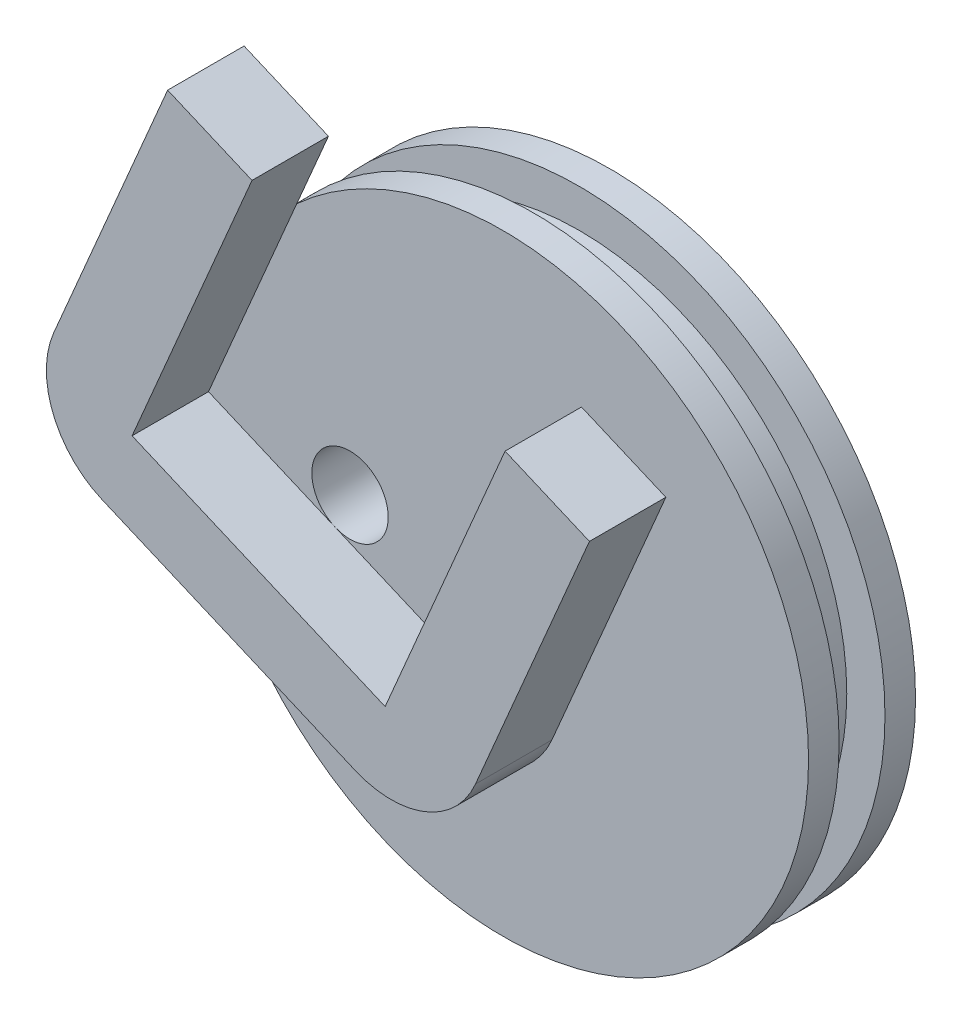
ISO-10303-21;
HEADER;
FILE_DESCRIPTION(('STEP AP214'),'2;1');
FILE_NAME('part.step','',(''),(''),'','','');
FILE_SCHEMA(('AUTOMOTIVE_DESIGN { 1 0 10303 214 1 1 1 1 }'));
ENDSEC;
DATA;
#1=APPLICATION_CONTEXT('core data for automotive mechanical design processes');
#2=APPLICATION_PROTOCOL_DEFINITION('international standard','automotive_design',2000,#1);
#3=PRODUCT_CONTEXT('',#1,'mechanical');
#4=PRODUCT('Part','Part','',(#3));
#5=PRODUCT_RELATED_PRODUCT_CATEGORY('part','',(#4));
#6=PRODUCT_DEFINITION_FORMATION('','',#4);
#7=PRODUCT_DEFINITION_CONTEXT('part definition',#1,'design');
#8=PRODUCT_DEFINITION('design','',#6,#7);
#9=PRODUCT_DEFINITION_SHAPE('','',#8);
#10=(LENGTH_UNIT() NAMED_UNIT(*) SI_UNIT(.MILLI.,.METRE.));
#11=(NAMED_UNIT(*) PLANE_ANGLE_UNIT() SI_UNIT($,.RADIAN.));
#12=(NAMED_UNIT(*) SI_UNIT($,.STERADIAN.) SOLID_ANGLE_UNIT());
#13=UNCERTAINTY_MEASURE_WITH_UNIT(LENGTH_MEASURE(1.E-05),#10,'distance_accuracy_value','');
#14=(GEOMETRIC_REPRESENTATION_CONTEXT(3) GLOBAL_UNCERTAINTY_ASSIGNED_CONTEXT((#13)) GLOBAL_UNIT_ASSIGNED_CONTEXT((#10,
#11,#12)) REPRESENTATION_CONTEXT('',''));
#15=CARTESIAN_POINT('',(0.,0.,0.));
#16=DIRECTION('',(0.,0.,1.));
#17=DIRECTION('',(1.,0.,0.));
#18=AXIS2_PLACEMENT_3D('',#15,#16,#17);
#19=CARTESIAN_POINT('',(0.,0.,3.5));
#20=DIRECTION('',(0.,0.,-1.));
#21=DIRECTION('',(-1.,0.,0.));
#22=AXIS2_PLACEMENT_3D('',#19,#20,#21);
#23=CYLINDRICAL_SURFACE('',#22,20.);
#24=CARTESIAN_POINT('',(0.,0.,3.5));
#25=DIRECTION('',(0.,0.,1.));
#26=DIRECTION('',(1.,0.,0.));
#27=AXIS2_PLACEMENT_3D('',#24,#25,#26);
#28=CIRCLE('',#27,20.);
#29=CARTESIAN_POINT('',(-13.4841723935684,14.7708190314731,3.5));
#30=VERTEX_POINT('',#29);
#31=CARTESIAN_POINT('',(-19.5822117840181,-4.06656878041691,3.5));
#32=VERTEX_POINT('',#31);
#33=EDGE_CURVE('E229',#30,#32,#28,.T.);
#34=ORIENTED_EDGE('',*,*,#33,.F.);
#35=EDGE_CURVE('E226',#32,#30,#28,.T.);
#36=ORIENTED_EDGE('',*,*,#35,.F.);
#37=EDGE_LOOP('',(#34,#36));
#38=FACE_BOUND('',#37,.T.);
#39=CARTESIAN_POINT('',(0.,0.,1.5));
#40=DIRECTION('',(0.,0.,1.));
#41=DIRECTION('',(1.,0.,0.));
#42=AXIS2_PLACEMENT_3D('',#39,#40,#41);
#43=CIRCLE('',#42,20.);
#44=CARTESIAN_POINT('',(20.,0.,1.5));
#45=VERTEX_POINT('',#44);
#46=EDGE_CURVE('E212',#45,#45,#43,.T.);
#47=ORIENTED_EDGE('',*,*,#46,.T.);
#48=EDGE_LOOP('',(#47));
#49=FACE_BOUND('',#48,.T.);
#50=ADVANCED_FACE('F39',(#38,#49),#23,.T.);
#51=CARTESIAN_POINT('',(0.,0.,3.5));
#52=DIRECTION('',(0.,0.,1.));
#53=DIRECTION('',(1.,0.,0.));
#54=AXIS2_PLACEMENT_3D('',#51,#52,#53);
#55=PLANE('',#54);
#56=DIRECTION('',(0.39234033710411,0.919820123655181,0.));
#57=VECTOR('',#56,1.);
#58=CARTESIAN_POINT('',(-19.2592319556569,1.231512724799,3.5));
#59=LINE('',#58,#57);
#60=CARTESIAN_POINT('',(-19.2592319556569,1.231512724799,3.5));
#61=VERTEX_POINT('',#60);
#62=EDGE_CURVE('E60',#61,#30,#59,.T.);
#63=ORIENTED_EDGE('',*,*,#62,.F.);
#64=DIRECTION('',(0.919820123655183,-0.392340337104106,0.));
#65=VECTOR('',#64,1.);
#66=CARTESIAN_POINT('',(-19.2592319556569,1.231512724799,3.5));
#67=LINE('',#66,#65);
#68=CARTESIAN_POINT('',(-10.9808508427603,-2.29955030913796,3.5));
#69=VERTEX_POINT('',#68);
#70=EDGE_CURVE('E49',#61,#69,#67,.T.);
#71=ORIENTED_EDGE('',*,*,#70,.T.);
#72=CARTESIAN_POINT('',(-10.,0.,3.5));
#73=DIRECTION('',(0.,0.,1.));
#74=DIRECTION('',(1.,0.,0.));
#75=AXIS2_PLACEMENT_3D('',#72,#73,#74);
#76=CIRCLE('',#75,2.5);
#77=EDGE_CURVE('E192',#69,#69,#76,.T.);
#78=ORIENTED_EDGE('',*,*,#77,.F.);
#79=CARTESIAN_POINT('',(-2.70246972986364,-5.8306133430749,3.5));
#80=VERTEX_POINT('',#79);
#81=EDGE_CURVE('E11',#69,#80,#67,.T.);
#82=ORIENTED_EDGE('',*,*,#81,.T.);
#83=DIRECTION('',(0.392340337104111,0.919820123655181,0.));
#84=VECTOR('',#83,1.);
#85=CARTESIAN_POINT('',(-2.70246972986364,-5.8306133430749,3.5));
#86=LINE('',#85,#84);
#87=CARTESIAN_POINT('',(5.14433701221858,12.5657891300287,3.5));
#88=VERTEX_POINT('',#87);
#89=EDGE_CURVE('E182',#80,#88,#86,.T.);
#90=ORIENTED_EDGE('',*,*,#89,.T.);
#91=DIRECTION('',(0.919820123655182,-0.392340337104108,0.));
#92=VECTOR('',#91,1.);
#93=CARTESIAN_POINT('',(5.14433701221858,12.5657891300287,3.5));
#94=LINE('',#93,#92);
#95=CARTESIAN_POINT('',(10.6632577541501,10.2117471074039,3.5));
#96=VERTEX_POINT('',#95);
#97=EDGE_CURVE('E181',#88,#96,#94,.T.);
#98=ORIENTED_EDGE('',*,*,#97,.T.);
#99=DIRECTION('',(0.392340337104132,0.919820123655172,0.));
#100=VECTOR('',#99,1.);
#101=CARTESIAN_POINT('',(3.20879134917148,-7.2648352420445,3.5));
#102=LINE('',#101,#100);
#103=CARTESIAN_POINT('',(3.2087913491715,-7.26483524204451,3.5));
#104=VERTEX_POINT('',#103);
#105=EDGE_CURVE('E183',#104,#96,#102,.T.);
#106=ORIENTED_EDGE('',*,*,#105,.F.);
#107=CARTESIAN_POINT('',(-2.31012939275951,-4.91079321941972,3.5));
#108=DIRECTION('',(0.,0.,1.));
#109=DIRECTION('',(1.,0.,0.));
#110=AXIS2_PLACEMENT_3D('',#107,#108,#109);
#111=CIRCLE('',#110,5.99999999999998);
#112=CARTESIAN_POINT('',(-4.66417141538418,-10.4297139613508,3.5));
#113=VERTEX_POINT('',#112);
#114=EDGE_CURVE('E153',#113,#104,#111,.T.);
#115=ORIENTED_EDGE('',*,*,#114,.F.);
#116=DIRECTION('',(0.919820123655183,-0.392340337104106,0.));
#117=VECTOR('',#116,1.);
#118=CARTESIAN_POINT('',(-21.2209336411774,-3.36758789347694,3.5));
#119=LINE('',#118,#117);
#120=EDGE_CURVE('E48',#32,#113,#119,.T.);
#121=ORIENTED_EDGE('',*,*,#120,.F.);
#122=ORIENTED_EDGE('',*,*,#35,.T.);
#123=EDGE_LOOP('',(#63,#71,#78,#82,#90,#98,#106,#115,#121,#122));
#124=FACE_BOUND('',#123,.T.);
#125=ADVANCED_FACE('F233',(#124),#55,.T.);
#126=CARTESIAN_POINT('',(0.,20.,1.5));
#127=DIRECTION('',(0.,0.,-1.));
#128=DIRECTION('',(-1.,0.,0.));
#129=AXIS2_PLACEMENT_3D('',#126,#127,#128);
#130=PLANE('',#129);
#131=CARTESIAN_POINT('',(0.,0.,1.5));
#132=DIRECTION('',(0.,0.,1.));
#133=DIRECTION('',(1.,0.,0.));
#134=AXIS2_PLACEMENT_3D('',#131,#132,#133);
#135=CIRCLE('',#134,17.5);
#136=CARTESIAN_POINT('',(17.5,0.,1.5));
#137=VERTEX_POINT('',#136);
#138=EDGE_CURVE('E224',#137,#137,#135,.T.);
#139=ORIENTED_EDGE('',*,*,#138,.T.);
#140=EDGE_LOOP('',(#139));
#141=FACE_BOUND('',#140,.T.);
#142=ORIENTED_EDGE('',*,*,#46,.F.);
#143=EDGE_LOOP('',(#142));
#144=FACE_BOUND('',#143,.T.);
#145=ADVANCED_FACE('F280',(#141,#144),#130,.T.);
#146=CARTESIAN_POINT('',(0.,0.,14.756637322569));
#147=DIRECTION('',(0.,0.,1.));
#148=DIRECTION('',(1.,0.,0.));
#149=AXIS2_PLACEMENT_3D('',#146,#147,#148);
#150=CYLINDRICAL_SURFACE('',#149,17.5);
#151=CARTESIAN_POINT('',(0.,0.,-1.5));
#152=DIRECTION('',(0.,0.,1.));
#153=DIRECTION('',(1.,0.,0.));
#154=AXIS2_PLACEMENT_3D('',#151,#152,#153);
#155=CIRCLE('',#154,17.5);
#156=CARTESIAN_POINT('',(17.5,0.,-1.5));
#157=VERTEX_POINT('',#156);
#158=EDGE_CURVE('E219',#157,#157,#155,.T.);
#159=ORIENTED_EDGE('',*,*,#158,.T.);
#160=EDGE_LOOP('',(#159));
#161=FACE_BOUND('',#160,.T.);
#162=ORIENTED_EDGE('',*,*,#138,.F.);
#163=EDGE_LOOP('',(#162));
#164=FACE_BOUND('',#163,.T.);
#165=ADVANCED_FACE('F269',(#161,#164),#150,.T.);
#166=CARTESIAN_POINT('',(0.,20.,-1.5));
#167=DIRECTION('',(0.,0.,-1.));
#168=DIRECTION('',(-1.,0.,0.));
#169=AXIS2_PLACEMENT_3D('',#166,#167,#168);
#170=PLANE('',#169);
#171=ORIENTED_EDGE('',*,*,#158,.F.);
#172=EDGE_LOOP('',(#171));
#173=FACE_BOUND('',#172,.T.);
#174=CARTESIAN_POINT('',(0.,0.,-1.5));
#175=DIRECTION('',(0.,0.,1.));
#176=DIRECTION('',(1.,0.,0.));
#177=AXIS2_PLACEMENT_3D('',#174,#175,#176);
#178=CIRCLE('',#177,20.);
#179=CARTESIAN_POINT('',(20.,0.,-1.5));
#180=VERTEX_POINT('',#179);
#181=EDGE_CURVE('E220',#180,#180,#178,.T.);
#182=ORIENTED_EDGE('',*,*,#181,.T.);
#183=EDGE_LOOP('',(#182));
#184=FACE_BOUND('',#183,.T.);
#185=ADVANCED_FACE('F263',(#173,#184),#170,.F.);
#186=CARTESIAN_POINT('',(0.,0.,-3.5));
#187=DIRECTION('',(0.,0.,1.));
#188=DIRECTION('',(1.,0.,0.));
#189=AXIS2_PLACEMENT_3D('',#186,#187,#188);
#190=PLANE('',#189);
#191=CARTESIAN_POINT('',(-10.,0.,-3.5));
#192=DIRECTION('',(0.,0.,1.));
#193=DIRECTION('',(1.,0.,0.));
#194=AXIS2_PLACEMENT_3D('',#191,#192,#193);
#195=CIRCLE('',#194,2.5);
#196=CARTESIAN_POINT('',(-7.5,0.,-3.5));
#197=VERTEX_POINT('',#196);
#198=EDGE_CURVE('E43',#197,#197,#195,.T.);
#199=ORIENTED_EDGE('',*,*,#198,.T.);
#200=EDGE_LOOP('',(#199));
#201=FACE_BOUND('',#200,.T.);
#202=CARTESIAN_POINT('',(0.,0.,-3.5));
#203=DIRECTION('',(0.,0.,1.));
#204=DIRECTION('',(1.,0.,0.));
#205=AXIS2_PLACEMENT_3D('',#202,#203,#204);
#206=CIRCLE('',#205,20.);
#207=CARTESIAN_POINT('',(20.,0.,-3.5));
#208=VERTEX_POINT('',#207);
#209=EDGE_CURVE('E227',#208,#208,#206,.T.);
#210=ORIENTED_EDGE('',*,*,#209,.F.);
#211=EDGE_LOOP('',(#210));
#212=FACE_BOUND('',#211,.T.);
#213=ADVANCED_FACE('F257',(#201,#212),#190,.F.);
#214=ORIENTED_EDGE('',*,*,#181,.F.);
#215=EDGE_LOOP('',(#214));
#216=FACE_BOUND('',#215,.T.);
#217=ORIENTED_EDGE('',*,*,#209,.T.);
#218=EDGE_LOOP('',(#217));
#219=FACE_BOUND('',#218,.T.);
#220=ADVANCED_FACE('F41',(#216,#219),#23,.T.);
#221=CARTESIAN_POINT('',(-10.,0.,-43.5));
#222=DIRECTION('',(0.,0.,1.));
#223=DIRECTION('',(1.,0.,0.));
#224=AXIS2_PLACEMENT_3D('',#221,#222,#223);
#225=CYLINDRICAL_SURFACE('',#224,2.5);
#226=ORIENTED_EDGE('',*,*,#77,.T.);
#227=EDGE_LOOP('',(#226));
#228=FACE_BOUND('',#227,.T.);
#229=ORIENTED_EDGE('',*,*,#198,.F.);
#230=EDGE_LOOP('',(#229));
#231=FACE_BOUND('',#230,.T.);
#232=ADVANCED_FACE('F251',(#228,#231),#225,.F.);
#233=CARTESIAN_POINT('',(-18.8668916185528,2.15133284845418,8.5));
#234=DIRECTION('',(0.,0.,-1.));
#235=DIRECTION('',(-1.,0.,0.));
#236=AXIS2_PLACEMENT_3D('',#233,#234,#235);
#237=CYLINDRICAL_SURFACE('',#236,6.00000000000002);
#238=CARTESIAN_POINT('',(-18.8668916185528,2.15133284845418,3.5));
#239=DIRECTION('',(0.,0.,-1.));
#240=DIRECTION('',(-1.,0.,0.));
#241=AXIS2_PLACEMENT_3D('',#238,#239,#240);
#242=CIRCLE('',#241,6.00000000000002);
#243=CARTESIAN_POINT('',(-21.2209336411774,-3.36758789347694,3.5));
#244=VERTEX_POINT('',#243);
#245=CARTESIAN_POINT('',(-24.3858123604839,4.505374871079,3.5));
#246=VERTEX_POINT('',#245);
#247=EDGE_CURVE('E175',#244,#246,#242,.T.);
#248=ORIENTED_EDGE('',*,*,#247,.F.);
#249=DIRECTION('',(0.,0.,-1.));
#250=VECTOR('',#249,1.);
#251=CARTESIAN_POINT('',(-21.2209336411774,-3.36758789347694,8.5));
#252=LINE('',#251,#250);
#253=CARTESIAN_POINT('',(-21.2209336411774,-3.36758789347694,8.5));
#254=VERTEX_POINT('',#253);
#255=EDGE_CURVE('E146',#254,#244,#252,.T.);
#256=ORIENTED_EDGE('',*,*,#255,.F.);
#257=CARTESIAN_POINT('',(-18.8668916185528,2.15133284845418,8.5));
#258=DIRECTION('',(0.,0.,-1.));
#259=DIRECTION('',(-1.,0.,0.));
#260=AXIS2_PLACEMENT_3D('',#257,#258,#259);
#261=CIRCLE('',#260,6.00000000000002);
#262=CARTESIAN_POINT('',(-24.3858123604839,4.505374871079,8.5));
#263=VERTEX_POINT('',#262);
#264=EDGE_CURVE('E141',#254,#263,#261,.T.);
#265=ORIENTED_EDGE('',*,*,#264,.T.);
#266=DIRECTION('',(0.,0.,-1.));
#267=VECTOR('',#266,1.);
#268=CARTESIAN_POINT('',(-24.3858123604839,4.505374871079,8.5));
#269=LINE('',#268,#267);
#270=EDGE_CURVE('E127',#263,#246,#269,.T.);
#271=ORIENTED_EDGE('',*,*,#270,.T.);
#272=EDGE_LOOP('',(#248,#256,#265,#271));
#273=FACE_BOUND('',#272,.T.);
#274=ADVANCED_FACE('F150',(#273),#237,.T.);
#275=CARTESIAN_POINT('',(-21.2209336411774,-3.36758789347694,8.5));
#276=DIRECTION('',(0.392340337104106,0.919820123655183,0.));
#277=DIRECTION('',(-0.919820123655183,0.392340337104106,0.));
#278=AXIS2_PLACEMENT_3D('',#275,#276,#277);
#279=PLANE('',#278);
#280=EDGE_CURVE('E147',#244,#32,#119,.T.);
#281=ORIENTED_EDGE('',*,*,#280,.T.);
#282=ORIENTED_EDGE('',*,*,#120,.T.);
#283=DIRECTION('',(0.,0.,-1.));
#284=VECTOR('',#283,1.);
#285=CARTESIAN_POINT('',(-4.66417141538418,-10.4297139613508,8.5));
#286=LINE('',#285,#284);
#287=CARTESIAN_POINT('',(-4.66417141538418,-10.4297139613508,8.5));
#288=VERTEX_POINT('',#287);
#289=EDGE_CURVE('E194',#288,#113,#286,.T.);
#290=ORIENTED_EDGE('',*,*,#289,.F.);
#291=DIRECTION('',(0.919820123655183,-0.392340337104106,0.));
#292=VECTOR('',#291,1.);
#293=CARTESIAN_POINT('',(-21.2209336411774,-3.36758789347694,8.5));
#294=LINE('',#293,#292);
#295=EDGE_CURVE('E139',#254,#288,#294,.T.);
#296=ORIENTED_EDGE('',*,*,#295,.F.);
#297=ORIENTED_EDGE('',*,*,#255,.T.);
#298=EDGE_LOOP('',(#281,#282,#290,#296,#297));
#299=FACE_BOUND('',#298,.T.);
#300=ADVANCED_FACE('F286',(#299),#279,.F.);
#301=CARTESIAN_POINT('',(-2.31012939275951,-4.91079321941972,8.5));
#302=DIRECTION('',(0.,0.,-1.));
#303=DIRECTION('',(-1.,0.,0.));
#304=AXIS2_PLACEMENT_3D('',#301,#302,#303);
#305=CYLINDRICAL_SURFACE('',#304,5.99999999999998);
#306=ORIENTED_EDGE('',*,*,#114,.T.);
#307=DIRECTION('',(0.,0.,-1.));
#308=VECTOR('',#307,1.);
#309=CARTESIAN_POINT('',(3.2087913491715,-7.26483524204451,8.5));
#310=LINE('',#309,#308);
#311=CARTESIAN_POINT('',(3.2087913491715,-7.26483524204451,8.5));
#312=VERTEX_POINT('',#311);
#313=EDGE_CURVE('E193',#312,#104,#310,.T.);
#314=ORIENTED_EDGE('',*,*,#313,.F.);
#315=CARTESIAN_POINT('',(-2.31012939275951,-4.91079321941972,8.5));
#316=DIRECTION('',(0.,0.,1.));
#317=DIRECTION('',(1.,0.,0.));
#318=AXIS2_PLACEMENT_3D('',#315,#316,#317);
#319=CIRCLE('',#318,5.99999999999998);
#320=EDGE_CURVE('E168',#288,#312,#319,.T.);
#321=ORIENTED_EDGE('',*,*,#320,.F.);
#322=ORIENTED_EDGE('',*,*,#289,.T.);
#323=EDGE_LOOP('',(#306,#314,#321,#322));
#324=FACE_BOUND('',#323,.T.);
#325=ADVANCED_FACE('F313',(#324),#305,.T.);
#326=CARTESIAN_POINT('',(3.20879134917148,-7.2648352420445,8.5));
#327=DIRECTION('',(-0.919820123655172,0.392340337104132,0.));
#328=DIRECTION('',(-0.392340337104132,-0.919820123655172,0.));
#329=AXIS2_PLACEMENT_3D('',#326,#327,#328);
#330=PLANE('',#329);
#331=ORIENTED_EDGE('',*,*,#105,.T.);
#332=DIRECTION('',(0.,0.,-1.));
#333=VECTOR('',#332,1.);
#334=CARTESIAN_POINT('',(10.6632577541501,10.2117471074039,8.5));
#335=LINE('',#334,#333);
#336=CARTESIAN_POINT('',(10.6632577541501,10.2117471074039,8.5));
#337=VERTEX_POINT('',#336);
#338=EDGE_CURVE('E196',#337,#96,#335,.T.);
#339=ORIENTED_EDGE('',*,*,#338,.F.);
#340=DIRECTION('',(0.392340337104132,0.919820123655172,0.));
#341=VECTOR('',#340,1.);
#342=CARTESIAN_POINT('',(3.20879134917148,-7.2648352420445,8.5));
#343=LINE('',#342,#341);
#344=EDGE_CURVE('E169',#312,#337,#343,.T.);
#345=ORIENTED_EDGE('',*,*,#344,.F.);
#346=ORIENTED_EDGE('',*,*,#313,.T.);
#347=EDGE_LOOP('',(#331,#339,#345,#346));
#348=FACE_BOUND('',#347,.T.);
#349=ADVANCED_FACE('F307',(#348),#330,.F.);
#350=CARTESIAN_POINT('',(5.14433701221858,12.5657891300287,8.5));
#351=DIRECTION('',(0.392340337104108,0.919820123655182,0.));
#352=DIRECTION('',(-0.919820123655182,0.392340337104108,0.));
#353=AXIS2_PLACEMENT_3D('',#350,#351,#352);
#354=PLANE('',#353);
#355=ORIENTED_EDGE('',*,*,#97,.F.);
#356=DIRECTION('',(0.,0.,-1.));
#357=VECTOR('',#356,1.);
#358=CARTESIAN_POINT('',(5.14433701221858,12.5657891300287,8.5));
#359=LINE('',#358,#357);
#360=CARTESIAN_POINT('',(5.14433701221858,12.5657891300287,8.5));
#361=VERTEX_POINT('',#360);
#362=EDGE_CURVE('E203',#361,#88,#359,.T.);
#363=ORIENTED_EDGE('',*,*,#362,.F.);
#364=DIRECTION('',(0.919820123655182,-0.392340337104108,0.));
#365=VECTOR('',#364,1.);
#366=CARTESIAN_POINT('',(5.14433701221858,12.5657891300287,8.5));
#367=LINE('',#366,#365);
#368=EDGE_CURVE('E164',#361,#337,#367,.T.);
#369=ORIENTED_EDGE('',*,*,#368,.T.);
#370=ORIENTED_EDGE('',*,*,#338,.T.);
#371=EDGE_LOOP('',(#355,#363,#369,#370));
#372=FACE_BOUND('',#371,.T.);
#373=ADVANCED_FACE('F305',(#372),#354,.T.);
#374=CARTESIAN_POINT('',(-2.70246972986364,-5.8306133430749,8.5));
#375=DIRECTION('',(-0.919820123655181,0.392340337104111,0.));
#376=DIRECTION('',(-0.392340337104111,-0.919820123655181,0.));
#377=AXIS2_PLACEMENT_3D('',#374,#375,#376);
#378=PLANE('',#377);
#379=ORIENTED_EDGE('',*,*,#89,.F.);
#380=DIRECTION('',(0.,0.,-1.));
#381=VECTOR('',#380,1.);
#382=CARTESIAN_POINT('',(-2.70246972986364,-5.8306133430749,8.5));
#383=LINE('',#382,#381);
#384=CARTESIAN_POINT('',(-2.70246972986364,-5.8306133430749,8.5));
#385=VERTEX_POINT('',#384);
#386=EDGE_CURVE('E204',#385,#80,#383,.T.);
#387=ORIENTED_EDGE('',*,*,#386,.F.);
#388=DIRECTION('',(0.392340337104111,0.919820123655181,0.));
#389=VECTOR('',#388,1.);
#390=CARTESIAN_POINT('',(-2.70246972986364,-5.8306133430749,8.5));
#391=LINE('',#390,#389);
#392=EDGE_CURVE('E165',#385,#361,#391,.T.);
#393=ORIENTED_EDGE('',*,*,#392,.T.);
#394=ORIENTED_EDGE('',*,*,#362,.T.);
#395=EDGE_LOOP('',(#379,#387,#393,#394));
#396=FACE_BOUND('',#395,.T.);
#397=ADVANCED_FACE('F298',(#396),#378,.T.);
#398=CARTESIAN_POINT('',(-19.2592319556569,1.231512724799,8.5));
#399=DIRECTION('',(0.392340337104106,0.919820123655183,0.));
#400=DIRECTION('',(-0.919820123655183,0.392340337104106,0.));
#401=AXIS2_PLACEMENT_3D('',#398,#399,#400);
#402=PLANE('',#401);
#403=ORIENTED_EDGE('',*,*,#70,.F.);
#404=DIRECTION('',(0.,0.,-1.));
#405=VECTOR('',#404,1.);
#406=CARTESIAN_POINT('',(-19.2592319556569,1.231512724799,8.5));
#407=LINE('',#406,#405);
#408=CARTESIAN_POINT('',(-19.2592319556569,1.231512724799,8.5));
#409=VERTEX_POINT('',#408);
#410=EDGE_CURVE('E206',#409,#61,#407,.T.);
#411=ORIENTED_EDGE('',*,*,#410,.F.);
#412=DIRECTION('',(0.919820123655183,-0.392340337104106,0.));
#413=VECTOR('',#412,1.);
#414=CARTESIAN_POINT('',(-19.2592319556569,1.231512724799,8.5));
#415=LINE('',#414,#413);
#416=EDGE_CURVE('E157',#409,#385,#415,.T.);
#417=ORIENTED_EDGE('',*,*,#416,.T.);
#418=ORIENTED_EDGE('',*,*,#386,.T.);
#419=ORIENTED_EDGE('',*,*,#81,.F.);
#420=EDGE_LOOP('',(#403,#411,#417,#418,#419));
#421=FACE_BOUND('',#420,.T.);
#422=ADVANCED_FACE('F253',(#421),#402,.T.);
#423=CARTESIAN_POINT('',(-19.2592319556569,1.231512724799,8.5));
#424=DIRECTION('',(-0.919820123655181,0.39234033710411,0.));
#425=DIRECTION('',(-0.39234033710411,-0.919820123655181,0.));
#426=AXIS2_PLACEMENT_3D('',#423,#424,#425);
#427=PLANE('',#426);
#428=ORIENTED_EDGE('',*,*,#62,.T.);
#429=CARTESIAN_POINT('',(-11.4124252135747,19.6279151979026,3.5));
#430=VERTEX_POINT('',#429);
#431=EDGE_CURVE('E176',#30,#430,#59,.T.);
#432=ORIENTED_EDGE('',*,*,#431,.T.);
#433=DIRECTION('',(0.,0.,-1.));
#434=VECTOR('',#433,1.);
#435=CARTESIAN_POINT('',(-11.4124252135747,19.6279151979026,8.5));
#436=LINE('',#435,#434);
#437=CARTESIAN_POINT('',(-11.4124252135747,19.6279151979026,8.5));
#438=VERTEX_POINT('',#437);
#439=EDGE_CURVE('E208',#438,#430,#436,.T.);
#440=ORIENTED_EDGE('',*,*,#439,.F.);
#441=DIRECTION('',(0.39234033710411,0.919820123655181,0.));
#442=VECTOR('',#441,1.);
#443=CARTESIAN_POINT('',(-19.2592319556569,1.231512724799,8.5));
#444=LINE('',#443,#442);
#445=EDGE_CURVE('E160',#409,#438,#444,.T.);
#446=ORIENTED_EDGE('',*,*,#445,.F.);
#447=ORIENTED_EDGE('',*,*,#410,.T.);
#448=EDGE_LOOP('',(#428,#432,#440,#446,#447));
#449=FACE_BOUND('',#448,.T.);
#450=ADVANCED_FACE('F247',(#449),#427,.F.);
#451=CARTESIAN_POINT('',(-16.9313459555054,21.9819572205271,8.5));
#452=DIRECTION('',(0.392340337104106,0.919820123655183,0.));
#453=DIRECTION('',(-0.919820123655183,0.392340337104106,0.));
#454=AXIS2_PLACEMENT_3D('',#451,#452,#453);
#455=PLANE('',#454);
#456=DIRECTION('',(0.919820123655183,-0.392340337104106,0.));
#457=VECTOR('',#456,1.);
#458=CARTESIAN_POINT('',(-16.9313459555054,21.9819572205271,3.5));
#459=LINE('',#458,#457);
#460=CARTESIAN_POINT('',(-16.9313459555054,21.9819572205271,3.5));
#461=VERTEX_POINT('',#460);
#462=EDGE_CURVE('E177',#461,#430,#459,.T.);
#463=ORIENTED_EDGE('',*,*,#462,.F.);
#464=DIRECTION('',(0.,0.,-1.));
#465=VECTOR('',#464,1.);
#466=CARTESIAN_POINT('',(-16.9313459555054,21.9819572205271,8.5));
#467=LINE('',#466,#465);
#468=CARTESIAN_POINT('',(-16.9313459555054,21.9819572205271,8.5));
#469=VERTEX_POINT('',#468);
#470=EDGE_CURVE('E137',#469,#461,#467,.T.);
#471=ORIENTED_EDGE('',*,*,#470,.F.);
#472=DIRECTION('',(0.919820123655183,-0.392340337104106,0.));
#473=VECTOR('',#472,1.);
#474=CARTESIAN_POINT('',(-16.9313459555054,21.9819572205271,8.5));
#475=LINE('',#474,#473);
#476=EDGE_CURVE('E144',#469,#438,#475,.T.);
#477=ORIENTED_EDGE('',*,*,#476,.T.);
#478=ORIENTED_EDGE('',*,*,#439,.T.);
#479=EDGE_LOOP('',(#463,#471,#477,#478));
#480=FACE_BOUND('',#479,.T.);
#481=ADVANCED_FACE('F295',(#480),#455,.T.);
#482=CARTESIAN_POINT('',(-24.3858123604839,4.505374871079,8.5));
#483=DIRECTION('',(-0.919820123655172,0.392340337104132,0.));
#484=DIRECTION('',(-0.392340337104132,-0.919820123655172,0.));
#485=AXIS2_PLACEMENT_3D('',#482,#483,#484);
#486=PLANE('',#485);
#487=DIRECTION('',(0.392340337104132,0.919820123655172,0.));
#488=VECTOR('',#487,1.);
#489=CARTESIAN_POINT('',(-24.3858123604839,4.505374871079,3.5));
#490=LINE('',#489,#488);
#491=EDGE_CURVE('E132',#246,#461,#490,.T.);
#492=ORIENTED_EDGE('',*,*,#491,.F.);
#493=ORIENTED_EDGE('',*,*,#270,.F.);
#494=DIRECTION('',(0.392340337104132,0.919820123655172,0.));
#495=VECTOR('',#494,1.);
#496=CARTESIAN_POINT('',(-24.3858123604839,4.505374871079,8.5));
#497=LINE('',#496,#495);
#498=EDGE_CURVE('E129',#263,#469,#497,.T.);
#499=ORIENTED_EDGE('',*,*,#498,.T.);
#500=ORIENTED_EDGE('',*,*,#470,.T.);
#501=EDGE_LOOP('',(#492,#493,#499,#500));
#502=FACE_BOUND('',#501,.T.);
#503=ADVANCED_FACE('F126',(#502),#486,.T.);
#504=CARTESIAN_POINT('',(-18.8668916185528,2.15133284845418,8.5));
#505=DIRECTION('',(0.,0.,-1.));
#506=DIRECTION('',(-1.,0.,0.));
#507=AXIS2_PLACEMENT_3D('',#504,#505,#506);
#508=PLANE('',#507);
#509=ORIENTED_EDGE('',*,*,#264,.F.);
#510=ORIENTED_EDGE('',*,*,#295,.T.);
#511=ORIENTED_EDGE('',*,*,#320,.T.);
#512=ORIENTED_EDGE('',*,*,#344,.T.);
#513=ORIENTED_EDGE('',*,*,#368,.F.);
#514=ORIENTED_EDGE('',*,*,#392,.F.);
#515=ORIENTED_EDGE('',*,*,#416,.F.);
#516=ORIENTED_EDGE('',*,*,#445,.T.);
#517=ORIENTED_EDGE('',*,*,#476,.F.);
#518=ORIENTED_EDGE('',*,*,#498,.F.);
#519=EDGE_LOOP('',(#509,#510,#511,#512,#513,#514,#515,#516,#517,#518));
#520=FACE_BOUND('',#519,.T.);
#521=ADVANCED_FACE('F142',(#520),#508,.F.);
#522=CARTESIAN_POINT('',(-18.8668916185528,2.15133284845418,3.5));
#523=DIRECTION('',(0.,0.,-1.));
#524=DIRECTION('',(-1.,0.,0.));
#525=AXIS2_PLACEMENT_3D('',#522,#523,#524);
#526=PLANE('',#525);
#527=ORIENTED_EDGE('',*,*,#431,.F.);
#528=ORIENTED_EDGE('',*,*,#33,.T.);
#529=ORIENTED_EDGE('',*,*,#280,.F.);
#530=ORIENTED_EDGE('',*,*,#247,.T.);
#531=ORIENTED_EDGE('',*,*,#491,.T.);
#532=ORIENTED_EDGE('',*,*,#462,.T.);
#533=EDGE_LOOP('',(#527,#528,#529,#530,#531,#532));
#534=FACE_BOUND('',#533,.T.);
#535=ADVANCED_FACE('F244',(#534),#526,.T.);
#536=CLOSED_SHELL('',(#50,#125,#145,#165,#185,#213,#220,#232,#274,#300,#325,#349,#373,#397,#422,
#450,#481,#503,#521,#535));
#537=MANIFOLD_SOLID_BREP('B2',#536);
#538=ADVANCED_BREP_SHAPE_REPRESENTATION('',(#18,#537),#14);
#539=SHAPE_DEFINITION_REPRESENTATION(#9,#538);
ENDSEC;
END-ISO-10303-21;
